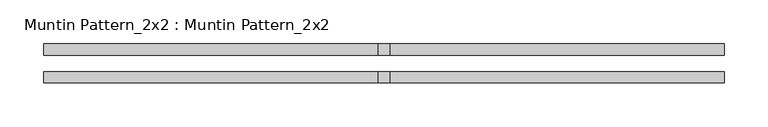
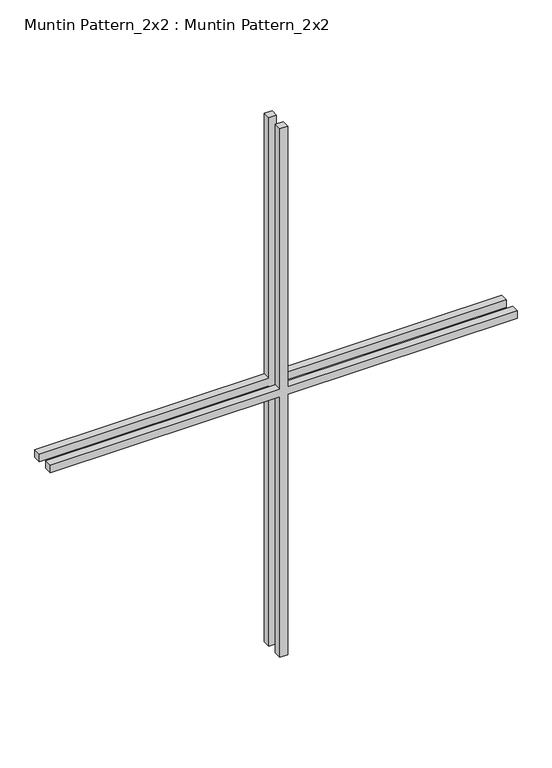
"""IFC4 building model written with IfcOpenShell, lengths in millimetres: proxy geometry, Muntin Pattern_2x2 : Muntin Pattern_2x2."""

from ifc_helpers import new_model, si_unit, frame, origin, place, context, project, spatial, polyline, outline, extrude, source, transform, mapped, element, save


def muntin_pattern_2x2_muntin_pattern_2x2_5e50c346(model_context):
    return source(origin(), model_context, "Body", "SweptSolid", [
        extrude(outline(polyline([(469.9, -6.35), (469.9, -387.35), (457.2, -387.35), (457.2, -6.35), (0.0, -6.35), (0.0, 6.35), (457.2, 6.35), (457.2, 387.35), (469.9, 387.35), (469.9, 6.35), (927.1, 6.35), (927.1, -6.35), (469.9, -6.35)])), frame((0.0, -22.225, 0.0), z_axis=(0.0, 1.0, 0.0), x_axis=(0.0, 0.0, 1.0)), (0.0, 0.0, 1.0), 12.7),
        extrude(outline(polyline([(469.9, -6.35), (469.9, -387.35), (457.2, -387.35), (457.2, -6.35), (0.0, -6.35), (0.0, 6.35), (457.2, 6.35), (457.2, 387.35), (469.9, 387.35), (469.9, 6.35), (927.1, 6.35), (927.1, -6.35), (469.9, -6.35)])), frame((0.0, 9.525, 0.0), z_axis=(0.0, 1.0, 0.0), x_axis=(0.0, 0.0, 1.0)), (0.0, 0.0, 1.0), 12.7),
    ])


if __name__ == "__main__":
    model = new_model("IFC4")
    model_context = context("Model", 3, world=origin())
    ifc_project = project(units=[si_unit("LENGTHUNIT", "METRE", prefix="MILLI")], contexts=[model_context])
    site = spatial("IfcSite", under=ifc_project)
    building = spatial("IfcBuilding", under=site)
    placement = place(None, origin())
    muntin_pattern_2x2_muntin_pattern_2x2_shape = muntin_pattern_2x2_muntin_pattern_2x2_5e50c346(model_context)
    element("IfcBuildingElementProxy", 1, Name="Muntin Pattern_2x2 : Muntin Pattern_2x2", ObjectType="Muntin Pattern_2x2 : Muntin Pattern_2x2", at=placement, inside=building, context=model_context, shape_type="MappedRepresentation", body=[
        mapped(muntin_pattern_2x2_muntin_pattern_2x2_shape, transform((0.0, 0.0, 0.0), x_axis=(1.0, 0.0, 0.0), y_axis=(0.0, 1.0, 0.0), z_axis=(0.0, 0.0, 1.0))),
    ])
    save(model, "model.ifc")

# Revit data of these elements
# Type "Muntin Pattern_2x2 : Muntin Pattern_2x2"
#   Width [instance default] = 4' - 0"
#   Thickness = 0' - 0 1/2"
#   Height [instance default] = 4' - 0"
#   Distance = 0' - 0 3/4"
#   Interior Material [instance default] = none
#   Exterior Material [instance default] = none
#   Default Elevation = 0
# Element 1 (IfcBuildingElementProxy, "Muntin Pattern_2x2 : Muntin Pattern_2x2")
#   Width = 2' - 6 1/2"
#   Height = 3' - 0 1/2"
#   Interior Material = Wood - Stained
#   Exterior Material = Clad - White
#   Materials on its faces: "Clad - White", "Wood - Stained"
# Materials
#   "Clad - White": class "Wood", colour RGB 242 242 238, transparency 0, Cost = 0
#   "Wood - Stained": class "Wood", colour RGB 224 178 126, transparency 0, Cost = 0
